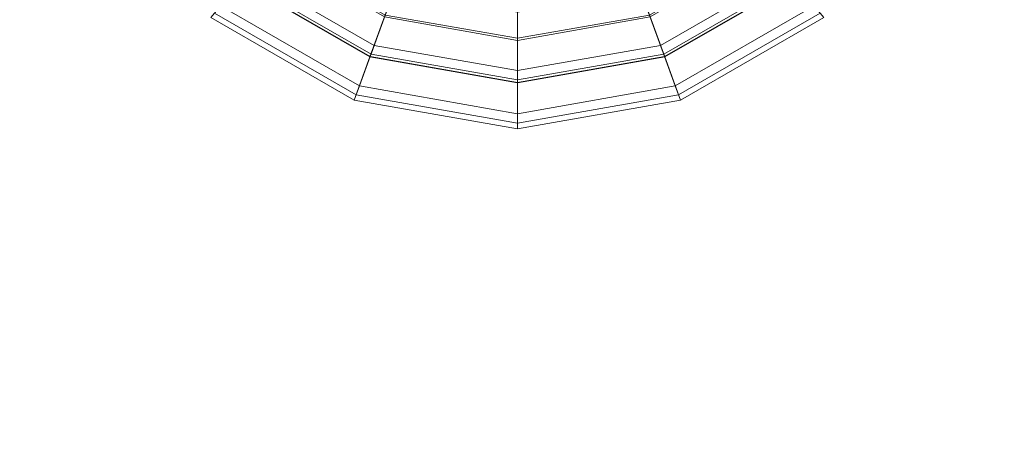
# Model space of a CAD drawing. Units: inches. Extents: x 375 to 1122, y 27 to 1069.
# Tile 127 of 155: x 720.668 to 723.463, y 900.211 to 901.45. Entities that reach past the tile are written whole.
import ezdxf

# ---------------------------------------------------------------- set-up
doc = ezdxf.new("R2010")
doc.units = ezdxf.units.IN
doc.layers.add('A-ANNO-DIMS', color=2, linetype='Continuous', lineweight=18)
doc.layers.add('Furniture', color=30, linetype='Continuous', lineweight=18)
doc.styles.get("Standard").update_dxf_attribs({"font": 'arial.ttf'})
doc.dimstyles.new('ISO-25', dxfattribs={"dimtxt": 12, "dimasz": 2.5, "dimexe": 1.5, "dimexo": 1.5, "dimtad": 1, "dimdec": 1, "dimlunit": 3, "dimtxsty": 'Standard', "dimblk": 'ARCHTICK', "dimcen": 2.5, "dimadec": 0, "dimazin": 0, "dimtfac": 1, "dimtdec": 1, "dimtmove": 0, "dimatfit": 3, "dimfxl": 1.5, "dimfxlon": 1, "dimarcsym": 0})

# ---------------------------------------------------------------- blocks, each defined once
blk = doc.blocks.new('A$C403C54AD')
for points in [[(0.927555, 0.939916, -0.042784), (0.895735, 0.928335, -0.039705), (0.895735, 0.928335, -0.039705), (0.921675, 0.950101, -0.042784)], [(0.924486, 0.938799, -0.039553), (0.927555, 0.939916, -0.042784), (0.921675, 0.950101, -0.042784), (0.919173, 0.948002, -0.039553)], [(0.926546, 0.939549, 0.078734), (0.921505, 0.937714, 0.060725), (0.916743, 0.945962, 0.060725), (0.920852, 0.949411, 0.078734)], [(0.924448, 0.938785, 0.1202), (0.92718, 0.93978, 0.106976), (0.921369, 0.949844, 0.106976), (0.919142, 0.947976, 0.1202)], [(0.92718, 0.93978, 0.106976), (0.926546, 0.939549, 0.078734), (0.920852, 0.949411, 0.078734), (0.921369, 0.949844, 0.106976)], [(0.909092, 0.933196, -0.036278), (0.924486, 0.938799, -0.039553), (0.919173, 0.948002, -0.039553), (0.906623, 0.937471, -0.036278)], [(0.919753, 0.937076, 0.129606), (0.924448, 0.938785, 0.1202), (0.919142, 0.947976, 0.1202), (0.915314, 0.944764, 0.129606)], [(0.918863, 0.936753, 0.062072), (0.923663, 0.9385, 0.079219), (0.918502, 0.947439, 0.079219), (0.914589, 0.944156, 0.062072)], [(0.924281, 0.938725, 0.106759), (0.921641, 0.937764, 0.119395), (0.916854, 0.946056, 0.119395), (0.919006, 0.947862, 0.106759)], [(0.923663, 0.9385, 0.079219), (0.924281, 0.938725, 0.106759), (0.919006, 0.947862, 0.106759), (0.918502, 0.947439, 0.079219)], [(0.929597, 0.928335, -0.042784), (0.895735, 0.928335, -0.039705), (0.895735, 0.928335, -0.039705), (0.927555, 0.939916, -0.042784)], [(0.928523, 0.928335, 0.078734), (0.923158, 0.928335, 0.060725), (0.921505, 0.937714, 0.060725), (0.926546, 0.939549, 0.078734)], [(0.926291, 0.928335, 0.1202), (0.929198, 0.928335, 0.106976), (0.92718, 0.93978, 0.106976), (0.924448, 0.938785, 0.1202)], [(0.926331, 0.928335, -0.039553), (0.929597, 0.928335, -0.042784), (0.927555, 0.939916, -0.042784), (0.924486, 0.938799, -0.039553)], [(0.929198, 0.928335, 0.106976), (0.928523, 0.928335, 0.078734), (0.926546, 0.939549, 0.078734), (0.92718, 0.93978, 0.106976)], [(0.909949, 0.928335, -0.036278), (0.926331, 0.928335, -0.039553), (0.924486, 0.938799, -0.039553), (0.909092, 0.933196, -0.036278)], [(0.920348, 0.928335, 0.062072), (0.925455, 0.928335, 0.079219), (0.923663, 0.9385, 0.079219), (0.918863, 0.936753, 0.062072)], [(0.921294, 0.928335, 0.129606), (0.926291, 0.928335, 0.1202), (0.924448, 0.938785, 0.1202), (0.919753, 0.937076, 0.129606)], [(0.926113, 0.928335, 0.106759), (0.923304, 0.928335, 0.119395), (0.921641, 0.937764, 0.119395), (0.924281, 0.938725, 0.106759)], [(0.925455, 0.928335, 0.079219), (0.926113, 0.928335, 0.106759), (0.924281, 0.938725, 0.106759), (0.923663, 0.9385, 0.079219)], [(0.923158, 0.928335, 0.060725), (0.916092, 0.928335, 0.050493), (0.914864, 0.935297, 0.050493), (0.921505, 0.937714, 0.060725)], [(0.923304, 0.928335, 0.119395), (0.918216, 0.928335, 0.129606), (0.91686, 0.936024, 0.129606), (0.921641, 0.937764, 0.119395)], [(0.927555, 0.916753, -0.042784), (0.895735, 0.928335, -0.039705), (0.895735, 0.928335, -0.039705), (0.929597, 0.928335, -0.042784)], [(0.921675, 0.906568, -0.042784), (0.895735, 0.928335, -0.039705), (0.895735, 0.928335, -0.039705), (0.927555, 0.916753, -0.042784)], [(0.909092, 0.923473, -0.036278), (0.924486, 0.91787, -0.039553), (0.926331, 0.928335, -0.039553), (0.909949, 0.928335, -0.036278)], [(0.921505, 0.918955, 0.060725), (0.914864, 0.921372, 0.050493), (0.916092, 0.928335, 0.050493), (0.923158, 0.928335, 0.060725)], [(0.921641, 0.918905, 0.119395), (0.91686, 0.920646, 0.129606), (0.918216, 0.928335, 0.129606), (0.923304, 0.928335, 0.119395)], [(0.918863, 0.919916, 0.062072), (0.923663, 0.918169, 0.079219), (0.925455, 0.928335, 0.079219), (0.920348, 0.928335, 0.062072)], [(0.919753, 0.919593, 0.129606), (0.924448, 0.917884, 0.1202), (0.926291, 0.928335, 0.1202), (0.921294, 0.928335, 0.129606)], [(0.926546, 0.91712, 0.078734), (0.921505, 0.918955, 0.060725), (0.923158, 0.928335, 0.060725), (0.928523, 0.928335, 0.078734)], [(0.924281, 0.917944, 0.106759), (0.921641, 0.918905, 0.119395), (0.923304, 0.928335, 0.119395), (0.926113, 0.928335, 0.106759)], [(0.923663, 0.918169, 0.079219), (0.924281, 0.917944, 0.106759), (0.926113, 0.928335, 0.106759), (0.925455, 0.928335, 0.079219)], [(0.924448, 0.917884, 0.1202), (0.92718, 0.916889, 0.106976), (0.929198, 0.928335, 0.106976), (0.926291, 0.928335, 0.1202)], [(0.924486, 0.91787, -0.039553), (0.927555, 0.916753, -0.042784), (0.929597, 0.928335, -0.042784), (0.926331, 0.928335, -0.039553)], [(0.92718, 0.916889, 0.106976), (0.926546, 0.91712, 0.078734), (0.928523, 0.928335, 0.078734), (0.929198, 0.928335, 0.106976)], [(0.906623, 0.919198, -0.036278), (0.919173, 0.908668, -0.039553), (0.924486, 0.91787, -0.039553), (0.909092, 0.923473, -0.036278)], [(0.914589, 0.912514, 0.062072), (0.918502, 0.90923, 0.079219), (0.923663, 0.918169, 0.079219), (0.918863, 0.919916, 0.062072)], [(0.915314, 0.911905, 0.129606), (0.919142, 0.908694, 0.1202), (0.924448, 0.917884, 0.1202), (0.919753, 0.919593, 0.129606)], [(0.920852, 0.907259, 0.078734), (0.916743, 0.910707, 0.060725), (0.921505, 0.918955, 0.060725), (0.926546, 0.91712, 0.078734)], [(0.919006, 0.908807, 0.106759), (0.916854, 0.910614, 0.119395), (0.921641, 0.918905, 0.119395), (0.924281, 0.917944, 0.106759)], [(0.918502, 0.90923, 0.079219), (0.919006, 0.908807, 0.106759), (0.924281, 0.917944, 0.106759), (0.923663, 0.918169, 0.079219)], [(0.919142, 0.908694, 0.1202), (0.921369, 0.906825, 0.106976), (0.92718, 0.916889, 0.106976), (0.924448, 0.917884, 0.1202)], [(0.919173, 0.908668, -0.039553), (0.921675, 0.906568, -0.042784), (0.927555, 0.916753, -0.042784), (0.924486, 0.91787, -0.039553)], [(0.921369, 0.906825, 0.106976), (0.920852, 0.907259, 0.078734), (0.926546, 0.91712, 0.078734), (0.92718, 0.916889, 0.106976)]]:
    blk.add_3dface(points)
blk = doc.blocks.new('_ArchTick')
at = {"color": 0, "linetype": 'ByBlock', "const_width": 0.15}
blk.add_lwpolyline([(-0.5, -0.5), (0.5, 0.5)], dxfattribs=at)
blk = doc.blocks.new('*D73')
at = {"layer": 'A-ANNO-DIMS', "color": 0, "lineweight": -2, "transparency": 16777216}
for p, q in [((686.7573, 932.4277), (686.7573, 929.4277)), ((770.7573, 932.4277), (770.7573, 929.4277)), ((686.7573, 930.9277), (770.7573, 930.9277)), ((770.7573, 930.9277), (987.6096, 930.9277))]:
    blk.add_line(p, q, dxfattribs=at)
at = {"layer": 'Defpoints', "color": 0, "transparency": 16777216}
for p in [(686.7573, 943.5277), (770.7573, 943.5277), (770.7573, 930.9277)]:
    blk.add_point(p, dxfattribs=at)
at = {"layer": 'A-ANNO-DIMS', "color": 0, "lineweight": -2, "transparency": 16777216, "xscale": 2.5, "yscale": 2.5, "zscale": 2.5, "rotation": 180}
blk.add_blockref('_ArchTick', (686.7573, 930.9277), dxfattribs=at)
at = {"layer": 'A-ANNO-DIMS', "color": 0, "lineweight": -2, "transparency": 16777216, "xscale": 2.5, "yscale": 2.5, "zscale": 2.5}
blk.add_blockref('_ArchTick', (770.7573, 930.9277), dxfattribs=at)
at = {"layer": 'A-ANNO-DIMS', "color": 0, "transparency": 16777216, "insert": (880.4335, 937.7573), "char_height": 12, "attachment_point": 5}
blk.add_mtext('2-PANEL SLIDER 7\'-0" TYP.', dxfattribs=at)

msp = doc.modelspace()

# ---------------------------------------------------------------- block references
at = {"layer": 'Furniture', "xscale": 39.9918517141215, "yscale": 39.9918517141215, "zscale": 39.9918517141215, "rotation": 270}
msp.add_blockref('A$C403C54AD', (684.9549, 938.3156, 0.024), dxfattribs=at)

# ---------------------------------------------------------------- dimensions: what is measured, and where the dimension line sits
at = {"layer": 'A-ANNO-DIMS'}
dim = msp.add_linear_dim(base=(770.7573, 930.9277), p1=(686.7573, 943.5277), p2=(770.7573, 943.5277), text='2-PANEL SLIDER <> TYP.', dimstyle='ISO-25', override={"dimdec": 1, "dimlfac": 1, "dimrnd": 0, "dimzin": 1, "dimdsep": 46, "dimlunit": 4, "dimfrac": 2}, dxfattribs=at)
dim.commit()
dim.dimension.update_dxf_attribs({"geometry": '*D73', "text_midpoint": (880.4335, 937.7573)})

doc.saveas('drawing.dxf')
